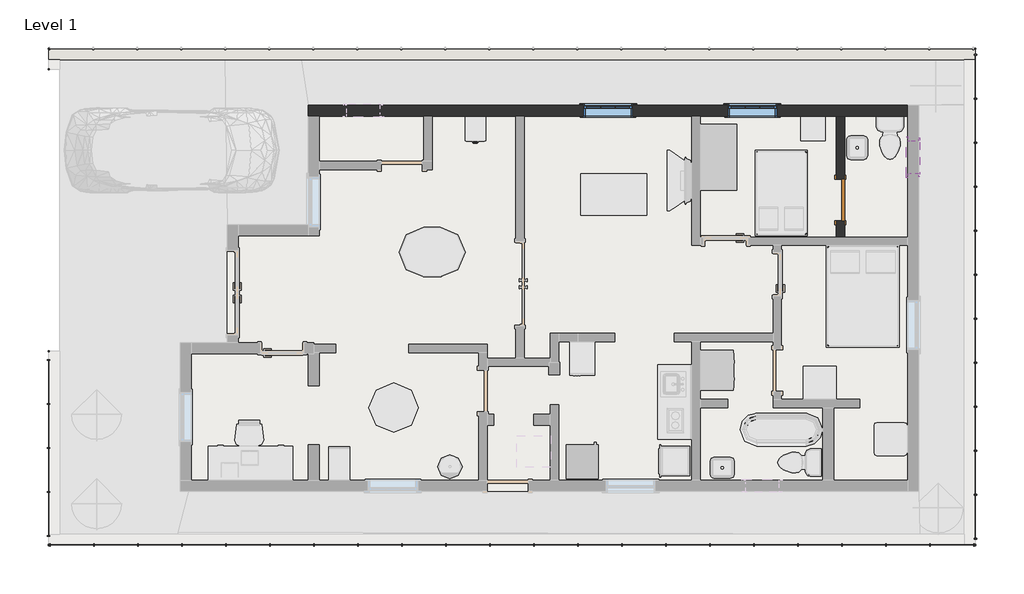
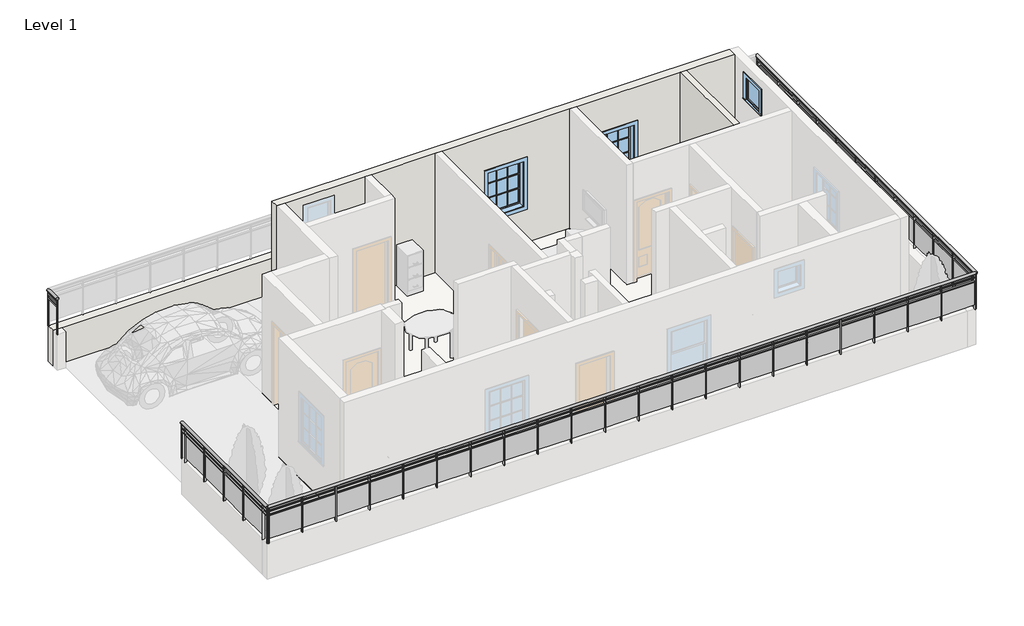
# One storey, part 2 of 3: 4 railings, 3 walls, 3 windows, 1 door, 1 slab.
"""IFC4 building model written with IfcOpenShell, lengths in millimetres."""

from ifc_helpers import new_model, si_unit, point, frame, origin, place, context, project, spatial, polyline, ellipse_curve, trimmed, outline, extrude, faceted_brep, transform, mapped, element, save
from ifc_brep_helpers import plane_surface, extruded_surface, advanced_brep
from components import door_059fdd7e, window_29c06734, window_e41d21a6

model = new_model("IFC4")

# Units and contexts
model_context = context("Model", 3, world=origin())
ifc_project = project(units=[si_unit("LENGTHUNIT", "METRE", prefix="MILLI")], contexts=[model_context])

# Site, building, storey
site = spatial("IfcSite", under=ifc_project)
building = spatial("IfcBuilding", under=site)
storey = spatial("IfcBuildingStorey", under=building, Name="Level 1", Elevation=0.0)

# Door
placement = place(None, origin())
door_shape = door_059fdd7e(model_context)
element("IfcDoor", 1, ObjectType="Single-Flush : 30\" x 80\"", at=placement, inside=storey, context=model_context, shape_type="MappedRepresentation", body=[
    mapped(door_shape, transform((-7474.6845566, 9582.2812219, 0.0), x_axis=(0.0, -1.0, 0.0), y_axis=(1.0, 0.0, 0.0), z_axis=(0.0, 0.0, 1.0))),
])

# Railings
element("IfcRailing", 2, ObjectType="Glass Panel - Bottom Fill", at=placement, inside=storey, context=model_context, shape_type="SolidModel", body=[
    advanced_brep(
    [(-22063.2202606, 6788.8658827, 1828.8), (-22139.4202606, 6788.8658827, 1828.8), (-22063.2202606, 3207.4658827, 1828.8), (-22139.4202606, 3207.4658827, 1828.8)],
    [
        (0, 1, ellipse_curve(frame((-22101.3202606, 6788.8658827, 1828.8), z_axis=(0.0, 1.0, 0.0), x_axis=(-1.0, 0.0, 0.0)), 38.1, 28.575)),
        (1, 0, ellipse_curve(frame((-22101.3202606, 6788.8658827, 1828.8), z_axis=(0.0, 1.0, 0.0), x_axis=(-1.0, 0.0, 0.0)), 38.1, 28.575)),
        (2, 3, ellipse_curve(frame((-22101.3202606, 3207.4658827, 1828.8), z_axis=(0.0, -1.0, 0.0), x_axis=(-1.0, 0.0, 0.0)), 38.1, 28.575)),
        (3, 2, ellipse_curve(frame((-22101.3202606, 3207.4658827, 1828.8), z_axis=(0.0, -1.0, 0.0), x_axis=(-1.0, 0.0, 0.0)), 38.1, 28.575)),
        (0, 2),
        (3, 1),
    ],
    [
        plane_surface(frame((-22101.3202606, 6788.8658827, 1828.8), z_axis=(0.0, 1.0, 0.0), x_axis=(0.0, 0.0, -1.0))),
        plane_surface(frame((-22101.3202606, 3207.4658827, 1828.8), z_axis=(0.0, -1.0, 0.0), x_axis=(0.0, 0.0, -1.0))),
        extruded_surface(trimmed(ellipse_curve(frame((-22101.3202606, 3207.4658827, 1828.8), z_axis=(0.0, 1.0, 0.0), x_axis=(-1.0, 0.0, 0.0)), 38.1, 28.575), [point((-22063.2202606, 3207.4658827, 1828.8))], [point((-22139.4202606, 3207.4658827, 1828.8))], True, "CARTESIAN"), (0.0, 3581.4, 0.0), 3581.4),
        extruded_surface(trimmed(ellipse_curve(frame((-22101.3202606, 3207.4658827, 1828.8), z_axis=(0.0, 1.0, 0.0), x_axis=(-1.0, 0.0, 0.0)), 38.1, 28.575), [point((-22139.4202606, 3207.4658827, 1828.8))], [point((-22063.2202606, 3207.4658827, 1828.8))], True, "CARTESIAN"), (0.0, 3581.4, 0.0), 3581.4),
    ],
    [
        (0, [[1, 2]]),
        (1, [[3, 4]]),
        (2, [[-1, 5, -4, 6]]),
        (3, [[-2, -6, -3, -5]]),
    ],
),
    extrude(outline(polyline([(-22114.0202606, 6788.8658827), (-22088.6202606, 6788.8658827), (-22088.6202606, 3207.4658827), (-22114.0202606, 3207.4658827), (-22114.0202606, 6788.8658827)])), frame((0.0, 0.0, 1714.5), z_axis=(0.0, 0.0, 1.0), x_axis=(1.0, 0.0, 0.0)), (0.0, 0.0, 1.0), 25.4),
    extrude(outline(polyline([(-22114.0202606, 6788.8658827), (-22088.6202606, 6788.8658827), (-22088.6202606, 3207.4658827), (-22114.0202606, 3207.4658827), (-22114.0202606, 6788.8658827)])), frame((0.0, 0.0, 1612.9), z_axis=(0.0, 0.0, 1.0), x_axis=(1.0, 0.0, 0.0)), (0.0, 0.0, 1.0), 25.4),
    extrude(outline(polyline([(-22126.7202606, 3378.9158827), (-22075.9202606, 3378.9158827), (-22075.9202606, 3366.2158827), (-22126.7202606, 3366.2158827), (-22126.7202606, 3378.9158827)])), frame((0.0, 0.0, 914.4), z_axis=(0.0, 0.0, 1.0), x_axis=(1.0, 0.0, 0.0)), (0.0, 0.0, 1.0), 885.6788223),
    extrude(outline(polyline([(-22094.7851036, 4185.3658827), (-22094.7851036, 3372.5658827), (-22101.1351036, 3372.5658827), (-22101.1351036, 4185.3658827), (-22094.7851036, 4185.3658827)])), frame((0.0, 0.0, 1016.0), z_axis=(0.0, 0.0, 1.0), x_axis=(1.0, 0.0, 0.0)), (0.0, 0.0, 1.0), 596.9),
    extrude(outline(polyline([(-22126.7202606, 4191.7158827), (-22075.9202606, 4191.7158827), (-22075.9202606, 4179.0158827), (-22126.7202606, 4179.0158827), (-22126.7202606, 4191.7158827)])), frame((0.0, 0.0, 914.4), z_axis=(0.0, 0.0, 1.0), x_axis=(1.0, 0.0, 0.0)), (0.0, 0.0, 1.0), 885.6788223),
    extrude(outline(polyline([(-22094.7851036, 4998.1658827), (-22094.7851036, 4185.3658827), (-22101.1351036, 4185.3658827), (-22101.1351036, 4998.1658827), (-22094.7851036, 4998.1658827)])), frame((0.0, 0.0, 1016.0), z_axis=(0.0, 0.0, 1.0), x_axis=(1.0, 0.0, 0.0)), (0.0, 0.0, 1.0), 596.9),
    extrude(outline(polyline([(-22126.7202606, 5004.5158827), (-22075.9202606, 5004.5158827), (-22075.9202606, 4991.8158827), (-22126.7202606, 4991.8158827), (-22126.7202606, 5004.5158827)])), frame((0.0, 0.0, 914.4), z_axis=(0.0, 0.0, 1.0), x_axis=(1.0, 0.0, 0.0)), (0.0, 0.0, 1.0), 885.6788223),
    extrude(outline(polyline([(-22094.7851036, 5810.9658827), (-22094.7851036, 4998.1658827), (-22101.1351036, 4998.1658827), (-22101.1351036, 5810.9658827), (-22094.7851036, 5810.9658827)])), frame((0.0, 0.0, 1016.0), z_axis=(0.0, 0.0, 1.0), x_axis=(1.0, 0.0, 0.0)), (0.0, 0.0, 1.0), 596.9),
    extrude(outline(polyline([(-22126.7202606, 5817.3158827), (-22075.9202606, 5817.3158827), (-22075.9202606, 5804.6158827), (-22126.7202606, 5804.6158827), (-22126.7202606, 5817.3158827)])), frame((0.0, 0.0, 914.4), z_axis=(0.0, 0.0, 1.0), x_axis=(1.0, 0.0, 0.0)), (0.0, 0.0, 1.0), 885.6788223),
    extrude(outline(polyline([(-22094.7851036, 6623.7658827), (-22094.7851036, 5810.9658827), (-22101.1351036, 5810.9658827), (-22101.1351036, 6623.7658827), (-22094.7851036, 6623.7658827)])), frame((0.0, 0.0, 1016.0), z_axis=(0.0, 0.0, 1.0), x_axis=(1.0, 0.0, 0.0)), (0.0, 0.0, 1.0), 596.9),
    extrude(outline(polyline([(-22126.7202606, 6630.1158827), (-22075.9202606, 6630.1158827), (-22075.9202606, 6617.4158827), (-22126.7202606, 6617.4158827), (-22126.7202606, 6630.1158827)])), frame((0.0, 0.0, 914.4), z_axis=(0.0, 0.0, 1.0), x_axis=(1.0, 0.0, 0.0)), (0.0, 0.0, 1.0), 885.6788223),
    extrude(outline(polyline([(-22110.8452606, 3220.1658827), (-22091.7952606, 3220.1658827), (-22091.7952606, 3201.1158827), (-22110.8452606, 3201.1158827), (-22110.8452606, 3220.1658827)])), frame((0.0, 0.0, 914.4), z_axis=(0.0, 0.0, 1.0), x_axis=(1.0, 0.0, 0.0)), (0.0, 0.0, 1.0), 885.6788223),
    extrude(outline(polyline([(-22110.8452606, 6795.2158827), (-22091.7952606, 6795.2158827), (-22091.7952606, 6776.1658827), (-22110.8452606, 6776.1658827), (-22110.8452606, 6795.2158827)])), frame((0.0, 0.0, 914.4), z_axis=(0.0, 0.0, 1.0), x_axis=(1.0, 0.0, 0.0)), (0.0, 0.0, 1.0), 885.6788223),
])
element("IfcRailing", 3, ObjectType="Glass Panel - Bottom Fill", at=placement, inside=storey, context=model_context, shape_type="SolidModel", body=[
    advanced_brep(
    [(-22101.3202606, 3245.5658827, 1828.8), (-22101.3202606, 3169.3658827, 1828.8), (-4981.7202606, 3245.5658827, 1828.8), (-4981.7202606, 3169.3658827, 1828.8)],
    [
        (0, 1, ellipse_curve(frame((-22101.3202606, 3207.4658827, 1828.8), z_axis=(-1.0, 0.0, 0.0), x_axis=(0.0, -1.0, 0.0)), 38.1, 28.575)),
        (1, 0, ellipse_curve(frame((-22101.3202606, 3207.4658827, 1828.8), z_axis=(-1.0, 0.0, 0.0), x_axis=(0.0, -1.0, 0.0)), 38.1, 28.575)),
        (2, 3, ellipse_curve(frame((-4981.7202606, 3207.4658827, 1828.8), z_axis=(1.0, 0.0, 0.0), x_axis=(0.0, -1.0, 0.0)), 38.1, 28.575)),
        (3, 2, ellipse_curve(frame((-4981.7202606, 3207.4658827, 1828.8), z_axis=(1.0, 0.0, 0.0), x_axis=(0.0, -1.0, 0.0)), 38.1, 28.575)),
        (0, 2),
        (3, 1),
    ],
    [
        plane_surface(frame((-22101.3202606, 3207.4658827, 1828.8), z_axis=(-1.0, 0.0, 0.0), x_axis=(0.0, 1.0, 0.0))),
        plane_surface(frame((-4981.7202606, 3207.4658827, 1828.8), z_axis=(1.0, 0.0, 0.0), x_axis=(0.0, 1.0, 0.0))),
        extruded_surface(trimmed(ellipse_curve(frame((-4981.7202606, 3207.4658827, 1828.8), z_axis=(-1.0, 0.0, 0.0), x_axis=(0.0, -1.0, 0.0)), 38.1, 28.575), [point((-4981.7202606, 3245.5658827, 1828.8))], [point((-4981.7202606, 3169.3658827, 1828.8))], True, "CARTESIAN"), (-17119.600000000002, 0.0, 0.0), 17119.600000000002),
        extruded_surface(trimmed(ellipse_curve(frame((-4981.7202606, 3207.4658827, 1828.8), z_axis=(-1.0, 0.0, 0.0), x_axis=(0.0, -1.0, 0.0)), 38.1, 28.575), [point((-4981.7202606, 3169.3658827, 1828.8))], [point((-4981.7202606, 3245.5658827, 1828.8))], True, "CARTESIAN"), (-17119.600000000002, 0.0, 0.0), 17119.600000000002),
    ],
    [
        (0, [[1, 2]]),
        (1, [[3, 4]]),
        (2, [[-1, 5, -4, 6]]),
        (3, [[-2, -6, -3, -5]]),
    ],
),
    extrude(outline(polyline([(-22101.3202606, 3194.7658827), (-22101.3202606, 3220.1658827), (-4981.7202606, 3220.1658827), (-4981.7202606, 3194.7658827), (-22101.3202606, 3194.7658827)])), frame((0.0, 0.0, 1714.5), z_axis=(0.0, 0.0, 1.0), x_axis=(1.0, 0.0, 0.0)), (0.0, 0.0, 1.0), 25.4),
    extrude(outline(polyline([(-22101.3202606, 3194.7658827), (-22101.3202606, 3220.1658827), (-4981.7202606, 3220.1658827), (-4981.7202606, 3194.7658827), (-22101.3202606, 3194.7658827)])), frame((0.0, 0.0, 1612.9), z_axis=(0.0, 0.0, 1.0), x_axis=(1.0, 0.0, 0.0)), (0.0, 0.0, 1.0), 25.4),
    extrude(outline(polyline([(-5013.4702606, 3182.0658827), (-5013.4702606, 3232.8658827), (-5000.7702606, 3232.8658827), (-5000.7702606, 3182.0658827), (-5013.4702606, 3182.0658827)])), frame((0.0, 0.0, 914.4), z_axis=(0.0, 0.0, 1.0), x_axis=(1.0, 0.0, 0.0)), (0.0, 0.0, 1.0), 885.6788223),
    extrude(outline(polyline([(-5819.9202606, 3214.0010397), (-5007.1202606, 3214.0010397), (-5007.1202606, 3207.6510397), (-5819.9202606, 3207.6510397), (-5819.9202606, 3214.0010397)])), frame((0.0, 0.0, 1016.0), z_axis=(0.0, 0.0, 1.0), x_axis=(1.0, 0.0, 0.0)), (0.0, 0.0, 1.0), 596.9),
    extrude(outline(polyline([(-5826.2702606, 3182.0658827), (-5826.2702606, 3232.8658827), (-5813.5702606, 3232.8658827), (-5813.5702606, 3182.0658827), (-5826.2702606, 3182.0658827)])), frame((0.0, 0.0, 914.4), z_axis=(0.0, 0.0, 1.0), x_axis=(1.0, 0.0, 0.0)), (0.0, 0.0, 1.0), 885.6788223),
    extrude(outline(polyline([(-6632.7202606, 3214.0010397), (-5819.9202606, 3214.0010397), (-5819.9202606, 3207.6510397), (-6632.7202606, 3207.6510397), (-6632.7202606, 3214.0010397)])), frame((0.0, 0.0, 1016.0), z_axis=(0.0, 0.0, 1.0), x_axis=(1.0, 0.0, 0.0)), (0.0, 0.0, 1.0), 596.9),
    extrude(outline(polyline([(-6639.0702606, 3182.0658827), (-6639.0702606, 3232.8658827), (-6626.3702606, 3232.8658827), (-6626.3702606, 3182.0658827), (-6639.0702606, 3182.0658827)])), frame((0.0, 0.0, 914.4), z_axis=(0.0, 0.0, 1.0), x_axis=(1.0, 0.0, 0.0)), (0.0, 0.0, 1.0), 885.6788223),
    extrude(outline(polyline([(-7445.5202606, 3214.0010397), (-6632.7202606, 3214.0010397), (-6632.7202606, 3207.6510397), (-7445.5202606, 3207.6510397), (-7445.5202606, 3214.0010397)])), frame((0.0, 0.0, 1016.0), z_axis=(0.0, 0.0, 1.0), x_axis=(1.0, 0.0, 0.0)), (0.0, 0.0, 1.0), 596.9),
    extrude(outline(polyline([(-7451.8702606, 3182.0658827), (-7451.8702606, 3232.8658827), (-7439.1702606, 3232.8658827), (-7439.1702606, 3182.0658827), (-7451.8702606, 3182.0658827)])), frame((0.0, 0.0, 914.4), z_axis=(0.0, 0.0, 1.0), x_axis=(1.0, 0.0, 0.0)), (0.0, 0.0, 1.0), 885.6788223),
    extrude(outline(polyline([(-8258.3202606, 3214.0010397), (-7445.5202606, 3214.0010397), (-7445.5202606, 3207.6510397), (-8258.3202606, 3207.6510397), (-8258.3202606, 3214.0010397)])), frame((0.0, 0.0, 1016.0), z_axis=(0.0, 0.0, 1.0), x_axis=(1.0, 0.0, 0.0)), (0.0, 0.0, 1.0), 596.9),
    extrude(outline(polyline([(-8264.6702606, 3182.0658827), (-8264.6702606, 3232.8658827), (-8251.9702606, 3232.8658827), (-8251.9702606, 3182.0658827), (-8264.6702606, 3182.0658827)])), frame((0.0, 0.0, 914.4), z_axis=(0.0, 0.0, 1.0), x_axis=(1.0, 0.0, 0.0)), (0.0, 0.0, 1.0), 885.6788223),
    extrude(outline(polyline([(-9071.1202606, 3214.0010397), (-8258.3202606, 3214.0010397), (-8258.3202606, 3207.6510397), (-9071.1202606, 3207.6510397), (-9071.1202606, 3214.0010397)])), frame((0.0, 0.0, 1016.0), z_axis=(0.0, 0.0, 1.0), x_axis=(1.0, 0.0, 0.0)), (0.0, 0.0, 1.0), 596.9),
    extrude(outline(polyline([(-9077.4702606, 3182.0658827), (-9077.4702606, 3232.8658827), (-9064.7702606, 3232.8658827), (-9064.7702606, 3182.0658827), (-9077.4702606, 3182.0658827)])), frame((0.0, 0.0, 914.4), z_axis=(0.0, 0.0, 1.0), x_axis=(1.0, 0.0, 0.0)), (0.0, 0.0, 1.0), 885.6788223),
    extrude(outline(polyline([(-9883.9202606, 3214.0010397), (-9071.1202606, 3214.0010397), (-9071.1202606, 3207.6510397), (-9883.9202606, 3207.6510397), (-9883.9202606, 3214.0010397)])), frame((0.0, 0.0, 1016.0), z_axis=(0.0, 0.0, 1.0), x_axis=(1.0, 0.0, 0.0)), (0.0, 0.0, 1.0), 596.9),
    extrude(outline(polyline([(-9890.2702606, 3182.0658827), (-9890.2702606, 3232.8658827), (-9877.5702606, 3232.8658827), (-9877.5702606, 3182.0658827), (-9890.2702606, 3182.0658827)])), frame((0.0, 0.0, 914.4), z_axis=(0.0, 0.0, 1.0), x_axis=(1.0, 0.0, 0.0)), (0.0, 0.0, 1.0), 885.6788223),
    extrude(outline(polyline([(-10696.7202606, 3214.0010397), (-9883.9202606, 3214.0010397), (-9883.9202606, 3207.6510397), (-10696.7202606, 3207.6510397), (-10696.7202606, 3214.0010397)])), frame((0.0, 0.0, 1016.0), z_axis=(0.0, 0.0, 1.0), x_axis=(1.0, 0.0, 0.0)), (0.0, 0.0, 1.0), 596.9),
    extrude(outline(polyline([(-10703.0702606, 3182.0658827), (-10703.0702606, 3232.8658827), (-10690.3702606, 3232.8658827), (-10690.3702606, 3182.0658827), (-10703.0702606, 3182.0658827)])), frame((0.0, 0.0, 914.4), z_axis=(0.0, 0.0, 1.0), x_axis=(1.0, 0.0, 0.0)), (0.0, 0.0, 1.0), 885.6788223),
    extrude(outline(polyline([(-11509.5202606, 3214.0010397), (-10696.7202606, 3214.0010397), (-10696.7202606, 3207.6510397), (-11509.5202606, 3207.6510397), (-11509.5202606, 3214.0010397)])), frame((0.0, 0.0, 1016.0), z_axis=(0.0, 0.0, 1.0), x_axis=(1.0, 0.0, 0.0)), (0.0, 0.0, 1.0), 596.9),
    extrude(outline(polyline([(-11515.8702606, 3182.0658827), (-11515.8702606, 3232.8658827), (-11503.1702606, 3232.8658827), (-11503.1702606, 3182.0658827), (-11515.8702606, 3182.0658827)])), frame((0.0, 0.0, 914.4), z_axis=(0.0, 0.0, 1.0), x_axis=(1.0, 0.0, 0.0)), (0.0, 0.0, 1.0), 885.6788223),
    extrude(outline(polyline([(-12322.3202606, 3214.0010397), (-11509.5202606, 3214.0010397), (-11509.5202606, 3207.6510397), (-12322.3202606, 3207.6510397), (-12322.3202606, 3214.0010397)])), frame((0.0, 0.0, 1016.0), z_axis=(0.0, 0.0, 1.0), x_axis=(1.0, 0.0, 0.0)), (0.0, 0.0, 1.0), 596.9),
    extrude(outline(polyline([(-12328.6702606, 3182.0658827), (-12328.6702606, 3232.8658827), (-12315.9702606, 3232.8658827), (-12315.9702606, 3182.0658827), (-12328.6702606, 3182.0658827)])), frame((0.0, 0.0, 914.4), z_axis=(0.0, 0.0, 1.0), x_axis=(1.0, 0.0, 0.0)), (0.0, 0.0, 1.0), 885.6788223),
    extrude(outline(polyline([(-13135.1202606, 3214.0010397), (-12322.3202606, 3214.0010397), (-12322.3202606, 3207.6510397), (-13135.1202606, 3207.6510397), (-13135.1202606, 3214.0010397)])), frame((0.0, 0.0, 1016.0), z_axis=(0.0, 0.0, 1.0), x_axis=(1.0, 0.0, 0.0)), (0.0, 0.0, 1.0), 596.9),
    extrude(outline(polyline([(-13141.4702606, 3182.0658827), (-13141.4702606, 3232.8658827), (-13128.7702606, 3232.8658827), (-13128.7702606, 3182.0658827), (-13141.4702606, 3182.0658827)])), frame((0.0, 0.0, 914.4), z_axis=(0.0, 0.0, 1.0), x_axis=(1.0, 0.0, 0.0)), (0.0, 0.0, 1.0), 885.6788223),
    extrude(outline(polyline([(-13947.9202606, 3214.0010397), (-13135.1202606, 3214.0010397), (-13135.1202606, 3207.6510397), (-13947.9202606, 3207.6510397), (-13947.9202606, 3214.0010397)])), frame((0.0, 0.0, 1016.0), z_axis=(0.0, 0.0, 1.0), x_axis=(1.0, 0.0, 0.0)), (0.0, 0.0, 1.0), 596.9),
    extrude(outline(polyline([(-13954.2702606, 3182.0658827), (-13954.2702606, 3232.8658827), (-13941.5702606, 3232.8658827), (-13941.5702606, 3182.0658827), (-13954.2702606, 3182.0658827)])), frame((0.0, 0.0, 914.4), z_axis=(0.0, 0.0, 1.0), x_axis=(1.0, 0.0, 0.0)), (0.0, 0.0, 1.0), 885.6788223),
    extrude(outline(polyline([(-14760.7202606, 3214.0010397), (-13947.9202606, 3214.0010397), (-13947.9202606, 3207.6510397), (-14760.7202606, 3207.6510397), (-14760.7202606, 3214.0010397)])), frame((0.0, 0.0, 1016.0), z_axis=(0.0, 0.0, 1.0), x_axis=(1.0, 0.0, 0.0)), (0.0, 0.0, 1.0), 596.9),
    extrude(outline(polyline([(-14767.0702606, 3182.0658827), (-14767.0702606, 3232.8658827), (-14754.3702606, 3232.8658827), (-14754.3702606, 3182.0658827), (-14767.0702606, 3182.0658827)])), frame((0.0, 0.0, 914.4), z_axis=(0.0, 0.0, 1.0), x_axis=(1.0, 0.0, 0.0)), (0.0, 0.0, 1.0), 885.6788223),
    extrude(outline(polyline([(-15573.5202606, 3214.0010397), (-14760.7202606, 3214.0010397), (-14760.7202606, 3207.6510397), (-15573.5202606, 3207.6510397), (-15573.5202606, 3214.0010397)])), frame((0.0, 0.0, 1016.0), z_axis=(0.0, 0.0, 1.0), x_axis=(1.0, 0.0, 0.0)), (0.0, 0.0, 1.0), 596.9),
    extrude(outline(polyline([(-15579.8702606, 3182.0658827), (-15579.8702606, 3232.8658827), (-15567.1702606, 3232.8658827), (-15567.1702606, 3182.0658827), (-15579.8702606, 3182.0658827)])), frame((0.0, 0.0, 914.4), z_axis=(0.0, 0.0, 1.0), x_axis=(1.0, 0.0, 0.0)), (0.0, 0.0, 1.0), 885.6788223),
    extrude(outline(polyline([(-16386.3202606, 3214.0010397), (-15573.5202606, 3214.0010397), (-15573.5202606, 3207.6510397), (-16386.3202606, 3207.6510397), (-16386.3202606, 3214.0010397)])), frame((0.0, 0.0, 1016.0), z_axis=(0.0, 0.0, 1.0), x_axis=(1.0, 0.0, 0.0)), (0.0, 0.0, 1.0), 596.9),
    extrude(outline(polyline([(-16392.6702606, 3182.0658827), (-16392.6702606, 3232.8658827), (-16379.9702606, 3232.8658827), (-16379.9702606, 3182.0658827), (-16392.6702606, 3182.0658827)])), frame((0.0, 0.0, 914.4), z_axis=(0.0, 0.0, 1.0), x_axis=(1.0, 0.0, 0.0)), (0.0, 0.0, 1.0), 885.6788223),
    extrude(outline(polyline([(-17199.1202606, 3214.0010397), (-16386.3202606, 3214.0010397), (-16386.3202606, 3207.6510397), (-17199.1202606, 3207.6510397), (-17199.1202606, 3214.0010397)])), frame((0.0, 0.0, 1016.0), z_axis=(0.0, 0.0, 1.0), x_axis=(1.0, 0.0, 0.0)), (0.0, 0.0, 1.0), 596.9),
    extrude(outline(polyline([(-17205.4702606, 3182.0658827), (-17205.4702606, 3232.8658827), (-17192.7702606, 3232.8658827), (-17192.7702606, 3182.0658827), (-17205.4702606, 3182.0658827)])), frame((0.0, 0.0, 914.4), z_axis=(0.0, 0.0, 1.0), x_axis=(1.0, 0.0, 0.0)), (0.0, 0.0, 1.0), 885.6788223),
    extrude(outline(polyline([(-18011.9202606, 3214.0010397), (-17199.1202606, 3214.0010397), (-17199.1202606, 3207.6510397), (-18011.9202606, 3207.6510397), (-18011.9202606, 3214.0010397)])), frame((0.0, 0.0, 1016.0), z_axis=(0.0, 0.0, 1.0), x_axis=(1.0, 0.0, 0.0)), (0.0, 0.0, 1.0), 596.9),
    extrude(outline(polyline([(-18018.2702606, 3182.0658827), (-18018.2702606, 3232.8658827), (-18005.5702606, 3232.8658827), (-18005.5702606, 3182.0658827), (-18018.2702606, 3182.0658827)])), frame((0.0, 0.0, 914.4), z_axis=(0.0, 0.0, 1.0), x_axis=(1.0, 0.0, 0.0)), (0.0, 0.0, 1.0), 885.6788223),
    extrude(outline(polyline([(-18824.7202606, 3214.0010397), (-18011.9202606, 3214.0010397), (-18011.9202606, 3207.6510397), (-18824.7202606, 3207.6510397), (-18824.7202606, 3214.0010397)])), frame((0.0, 0.0, 1016.0), z_axis=(0.0, 0.0, 1.0), x_axis=(1.0, 0.0, 0.0)), (0.0, 0.0, 1.0), 596.9),
    extrude(outline(polyline([(-18831.0702606, 3182.0658827), (-18831.0702606, 3232.8658827), (-18818.3702606, 3232.8658827), (-18818.3702606, 3182.0658827), (-18831.0702606, 3182.0658827)])), frame((0.0, 0.0, 914.4), z_axis=(0.0, 0.0, 1.0), x_axis=(1.0, 0.0, 0.0)), (0.0, 0.0, 1.0), 885.6788223),
    extrude(outline(polyline([(-19637.5202606, 3214.0010397), (-18824.7202606, 3214.0010397), (-18824.7202606, 3207.6510397), (-19637.5202606, 3207.6510397), (-19637.5202606, 3214.0010397)])), frame((0.0, 0.0, 1016.0), z_axis=(0.0, 0.0, 1.0), x_axis=(1.0, 0.0, 0.0)), (0.0, 0.0, 1.0), 596.9),
    extrude(outline(polyline([(-19643.8702606, 3182.0658827), (-19643.8702606, 3232.8658827), (-19631.1702606, 3232.8658827), (-19631.1702606, 3182.0658827), (-19643.8702606, 3182.0658827)])), frame((0.0, 0.0, 914.4), z_axis=(0.0, 0.0, 1.0), x_axis=(1.0, 0.0, 0.0)), (0.0, 0.0, 1.0), 885.6788223),
    extrude(outline(polyline([(-20450.3202606, 3214.0010397), (-19637.5202606, 3214.0010397), (-19637.5202606, 3207.6510397), (-20450.3202606, 3207.6510397), (-20450.3202606, 3214.0010397)])), frame((0.0, 0.0, 1016.0), z_axis=(0.0, 0.0, 1.0), x_axis=(1.0, 0.0, 0.0)), (0.0, 0.0, 1.0), 596.9),
    extrude(outline(polyline([(-20456.6702606, 3182.0658827), (-20456.6702606, 3232.8658827), (-20443.9702606, 3232.8658827), (-20443.9702606, 3182.0658827), (-20456.6702606, 3182.0658827)])), frame((0.0, 0.0, 914.4), z_axis=(0.0, 0.0, 1.0), x_axis=(1.0, 0.0, 0.0)), (0.0, 0.0, 1.0), 885.6788223),
    extrude(outline(polyline([(-21263.1202606, 3214.0010397), (-20450.3202606, 3214.0010397), (-20450.3202606, 3207.6510397), (-21263.1202606, 3207.6510397), (-21263.1202606, 3214.0010397)])), frame((0.0, 0.0, 1016.0), z_axis=(0.0, 0.0, 1.0), x_axis=(1.0, 0.0, 0.0)), (0.0, 0.0, 1.0), 596.9),
    extrude(outline(polyline([(-21269.4702606, 3182.0658827), (-21269.4702606, 3232.8658827), (-21256.7702606, 3232.8658827), (-21256.7702606, 3182.0658827), (-21269.4702606, 3182.0658827)])), frame((0.0, 0.0, 914.4), z_axis=(0.0, 0.0, 1.0), x_axis=(1.0, 0.0, 0.0)), (0.0, 0.0, 1.0), 885.6788223),
    extrude(outline(polyline([(-22075.9202606, 3214.0010397), (-21263.1202606, 3214.0010397), (-21263.1202606, 3207.6510397), (-22075.9202606, 3207.6510397), (-22075.9202606, 3214.0010397)])), frame((0.0, 0.0, 1016.0), z_axis=(0.0, 0.0, 1.0), x_axis=(1.0, 0.0, 0.0)), (0.0, 0.0, 1.0), 596.9),
    extrude(outline(polyline([(-22082.2702606, 3182.0658827), (-22082.2702606, 3232.8658827), (-22069.5702606, 3232.8658827), (-22069.5702606, 3182.0658827), (-22082.2702606, 3182.0658827)])), frame((0.0, 0.0, 914.4), z_axis=(0.0, 0.0, 1.0), x_axis=(1.0, 0.0, 0.0)), (0.0, 0.0, 1.0), 885.6788223),
    extrude(outline(polyline([(-4994.4202606, 3197.9408827), (-4994.4202606, 3216.9908827), (-4975.3702606, 3216.9908827), (-4975.3702606, 3197.9408827), (-4994.4202606, 3197.9408827)])), frame((0.0, 0.0, 914.4), z_axis=(0.0, 0.0, 1.0), x_axis=(1.0, 0.0, 0.0)), (0.0, 0.0, 1.0), 885.6788223),
    extrude(outline(polyline([(-22107.6702606, 3197.9408827), (-22107.6702606, 3216.9908827), (-22088.6202606, 3216.9908827), (-22088.6202606, 3197.9408827), (-22107.6702606, 3197.9408827)])), frame((0.0, 0.0, 914.4), z_axis=(0.0, 0.0, 1.0), x_axis=(1.0, 0.0, 0.0)), (0.0, 0.0, 1.0), 885.6788223),
])
element("IfcRailing", 4, ObjectType="Glass Panel - Bottom Fill", at=placement, inside=storey, context=model_context, shape_type="SolidModel", body=[
    advanced_brep(
    [(-5019.8202606, 3207.4658827, 1828.8), (-4943.6202606, 3207.4658827, 1828.8), (-5019.8202606, 12376.8658827, 1828.8), (-4943.6202606, 12376.8658827, 1828.8)],
    [
        (0, 1, ellipse_curve(frame((-4981.7202606, 3207.4658827, 1828.8), z_axis=(0.0, -1.0, 0.0), x_axis=(1.0, 0.0, 0.0)), 38.1, 28.575)),
        (1, 0, ellipse_curve(frame((-4981.7202606, 3207.4658827, 1828.8), z_axis=(0.0, -1.0, 0.0), x_axis=(1.0, 0.0, 0.0)), 38.1, 28.575)),
        (2, 3, ellipse_curve(frame((-4981.7202606, 12376.8658827, 1828.8), z_axis=(0.0, 1.0, 0.0), x_axis=(1.0, 0.0, 0.0)), 38.1, 28.575)),
        (3, 2, ellipse_curve(frame((-4981.7202606, 12376.8658827, 1828.8), z_axis=(0.0, 1.0, 0.0), x_axis=(1.0, 0.0, 0.0)), 38.1, 28.575)),
        (0, 2),
        (3, 1),
    ],
    [
        plane_surface(frame((-4981.7202606, 3207.4658827, 1828.8), z_axis=(0.0, -1.0, 0.0), x_axis=(0.0, 0.0, 1.0))),
        plane_surface(frame((-4981.7202606, 12376.8658827, 1828.8), z_axis=(0.0, 1.0, 0.0), x_axis=(0.0, 0.0, 1.0))),
        extruded_surface(trimmed(ellipse_curve(frame((-4981.7202606, 12376.8658827, 1828.8), z_axis=(0.0, -1.0, 0.0), x_axis=(1.0, 0.0, 0.0)), 38.1, 28.575), [point((-5019.8202606, 12376.8658827, 1828.8))], [point((-4943.6202606, 12376.8658827, 1828.8))], True, "CARTESIAN"), (0.0, -9169.4, 0.0), 9169.4),
        extruded_surface(trimmed(ellipse_curve(frame((-4981.7202606, 12376.8658827, 1828.8), z_axis=(0.0, -1.0, 0.0), x_axis=(1.0, 0.0, 0.0)), 38.1, 28.575), [point((-4943.6202606, 12376.8658827, 1828.8))], [point((-5019.8202606, 12376.8658827, 1828.8))], True, "CARTESIAN"), (0.0, -9169.4, 0.0), 9169.4),
    ],
    [
        (0, [[1, 2]]),
        (1, [[3, 4]]),
        (2, [[-1, 5, -4, 6]]),
        (3, [[-2, -6, -3, -5]]),
    ],
),
    extrude(outline(polyline([(-4969.0202606, 3207.4658827), (-4994.4202606, 3207.4658827), (-4994.4202606, 12376.8658827), (-4969.0202606, 12376.8658827), (-4969.0202606, 3207.4658827)])), frame((0.0, 0.0, 1714.5), z_axis=(0.0, 0.0, 1.0), x_axis=(1.0, 0.0, 0.0)), (0.0, 0.0, 1.0), 25.4),
    extrude(outline(polyline([(-4969.0202606, 3207.4658827), (-4994.4202606, 3207.4658827), (-4994.4202606, 12376.8658827), (-4969.0202606, 12376.8658827), (-4969.0202606, 3207.4658827)])), frame((0.0, 0.0, 1612.9), z_axis=(0.0, 0.0, 1.0), x_axis=(1.0, 0.0, 0.0)), (0.0, 0.0, 1.0), 25.4),
    extrude(outline(polyline([(-4956.3202606, 12256.2158827), (-5007.1202606, 12256.2158827), (-5007.1202606, 12268.9158827), (-4956.3202606, 12268.9158827), (-4956.3202606, 12256.2158827)])), frame((0.0, 0.0, 914.4), z_axis=(0.0, 0.0, 1.0), x_axis=(1.0, 0.0, 0.0)), (0.0, 0.0, 1.0), 885.6788223),
    extrude(outline(polyline([(-4988.2554176, 11449.7658827), (-4988.2554176, 12262.5658827), (-4981.9054176, 12262.5658827), (-4981.9054176, 11449.7658827), (-4988.2554176, 11449.7658827)])), frame((0.0, 0.0, 1016.0), z_axis=(0.0, 0.0, 1.0), x_axis=(1.0, 0.0, 0.0)), (0.0, 0.0, 1.0), 596.9),
    extrude(outline(polyline([(-4956.3202606, 11443.4158827), (-5007.1202606, 11443.4158827), (-5007.1202606, 11456.1158827), (-4956.3202606, 11456.1158827), (-4956.3202606, 11443.4158827)])), frame((0.0, 0.0, 914.4), z_axis=(0.0, 0.0, 1.0), x_axis=(1.0, 0.0, 0.0)), (0.0, 0.0, 1.0), 885.6788223),
    extrude(outline(polyline([(-4988.2554176, 10636.9658827), (-4988.2554176, 11449.7658827), (-4981.9054176, 11449.7658827), (-4981.9054176, 10636.9658827), (-4988.2554176, 10636.9658827)])), frame((0.0, 0.0, 1016.0), z_axis=(0.0, 0.0, 1.0), x_axis=(1.0, 0.0, 0.0)), (0.0, 0.0, 1.0), 596.9),
    extrude(outline(polyline([(-4956.3202606, 10630.6158827), (-5007.1202606, 10630.6158827), (-5007.1202606, 10643.3158827), (-4956.3202606, 10643.3158827), (-4956.3202606, 10630.6158827)])), frame((0.0, 0.0, 914.4), z_axis=(0.0, 0.0, 1.0), x_axis=(1.0, 0.0, 0.0)), (0.0, 0.0, 1.0), 885.6788223),
    extrude(outline(polyline([(-4988.2554176, 9824.1658827), (-4988.2554176, 10636.9658827), (-4981.9054176, 10636.9658827), (-4981.9054176, 9824.1658827), (-4988.2554176, 9824.1658827)])), frame((0.0, 0.0, 1016.0), z_axis=(0.0, 0.0, 1.0), x_axis=(1.0, 0.0, 0.0)), (0.0, 0.0, 1.0), 596.9),
    extrude(outline(polyline([(-4956.3202606, 9817.8158827), (-5007.1202606, 9817.8158827), (-5007.1202606, 9830.5158827), (-4956.3202606, 9830.5158827), (-4956.3202606, 9817.8158827)])), frame((0.0, 0.0, 914.4), z_axis=(0.0, 0.0, 1.0), x_axis=(1.0, 0.0, 0.0)), (0.0, 0.0, 1.0), 885.6788223),
    extrude(outline(polyline([(-4988.2554176, 9011.3658827), (-4988.2554176, 9824.1658827), (-4981.9054176, 9824.1658827), (-4981.9054176, 9011.3658827), (-4988.2554176, 9011.3658827)])), frame((0.0, 0.0, 1016.0), z_axis=(0.0, 0.0, 1.0), x_axis=(1.0, 0.0, 0.0)), (0.0, 0.0, 1.0), 596.9),
    extrude(outline(polyline([(-4956.3202606, 9005.0158827), (-5007.1202606, 9005.0158827), (-5007.1202606, 9017.7158827), (-4956.3202606, 9017.7158827), (-4956.3202606, 9005.0158827)])), frame((0.0, 0.0, 914.4), z_axis=(0.0, 0.0, 1.0), x_axis=(1.0, 0.0, 0.0)), (0.0, 0.0, 1.0), 885.6788223),
    extrude(outline(polyline([(-4988.2554176, 8198.5658827), (-4988.2554176, 9011.3658827), (-4981.9054176, 9011.3658827), (-4981.9054176, 8198.5658827), (-4988.2554176, 8198.5658827)])), frame((0.0, 0.0, 1016.0), z_axis=(0.0, 0.0, 1.0), x_axis=(1.0, 0.0, 0.0)), (0.0, 0.0, 1.0), 596.9),
    extrude(outline(polyline([(-4956.3202606, 8192.2158827), (-5007.1202606, 8192.2158827), (-5007.1202606, 8204.9158827), (-4956.3202606, 8204.9158827), (-4956.3202606, 8192.2158827)])), frame((0.0, 0.0, 914.4), z_axis=(0.0, 0.0, 1.0), x_axis=(1.0, 0.0, 0.0)), (0.0, 0.0, 1.0), 885.6788223),
    extrude(outline(polyline([(-4988.2554176, 7385.7658827), (-4988.2554176, 8198.5658827), (-4981.9054176, 8198.5658827), (-4981.9054176, 7385.7658827), (-4988.2554176, 7385.7658827)])), frame((0.0, 0.0, 1016.0), z_axis=(0.0, 0.0, 1.0), x_axis=(1.0, 0.0, 0.0)), (0.0, 0.0, 1.0), 596.9),
    extrude(outline(polyline([(-4956.3202606, 7379.4158827), (-5007.1202606, 7379.4158827), (-5007.1202606, 7392.1158827), (-4956.3202606, 7392.1158827), (-4956.3202606, 7379.4158827)])), frame((0.0, 0.0, 914.4), z_axis=(0.0, 0.0, 1.0), x_axis=(1.0, 0.0, 0.0)), (0.0, 0.0, 1.0), 885.6788223),
    extrude(outline(polyline([(-4988.2554176, 6572.9658827), (-4988.2554176, 7385.7658827), (-4981.9054176, 7385.7658827), (-4981.9054176, 6572.9658827), (-4988.2554176, 6572.9658827)])), frame((0.0, 0.0, 1016.0), z_axis=(0.0, 0.0, 1.0), x_axis=(1.0, 0.0, 0.0)), (0.0, 0.0, 1.0), 596.9),
    extrude(outline(polyline([(-4956.3202606, 6566.6158827), (-5007.1202606, 6566.6158827), (-5007.1202606, 6579.3158827), (-4956.3202606, 6579.3158827), (-4956.3202606, 6566.6158827)])), frame((0.0, 0.0, 914.4), z_axis=(0.0, 0.0, 1.0), x_axis=(1.0, 0.0, 0.0)), (0.0, 0.0, 1.0), 885.6788223),
    extrude(outline(polyline([(-4988.2554176, 5760.1658827), (-4988.2554176, 6572.9658827), (-4981.9054176, 6572.9658827), (-4981.9054176, 5760.1658827), (-4988.2554176, 5760.1658827)])), frame((0.0, 0.0, 1016.0), z_axis=(0.0, 0.0, 1.0), x_axis=(1.0, 0.0, 0.0)), (0.0, 0.0, 1.0), 596.9),
    extrude(outline(polyline([(-4956.3202606, 5753.8158827), (-5007.1202606, 5753.8158827), (-5007.1202606, 5766.5158827), (-4956.3202606, 5766.5158827), (-4956.3202606, 5753.8158827)])), frame((0.0, 0.0, 914.4), z_axis=(0.0, 0.0, 1.0), x_axis=(1.0, 0.0, 0.0)), (0.0, 0.0, 1.0), 885.6788223),
    extrude(outline(polyline([(-4988.2554176, 4947.3658827), (-4988.2554176, 5760.1658827), (-4981.9054176, 5760.1658827), (-4981.9054176, 4947.3658827), (-4988.2554176, 4947.3658827)])), frame((0.0, 0.0, 1016.0), z_axis=(0.0, 0.0, 1.0), x_axis=(1.0, 0.0, 0.0)), (0.0, 0.0, 1.0), 596.9),
    extrude(outline(polyline([(-4956.3202606, 4941.0158827), (-5007.1202606, 4941.0158827), (-5007.1202606, 4953.7158827), (-4956.3202606, 4953.7158827), (-4956.3202606, 4941.0158827)])), frame((0.0, 0.0, 914.4), z_axis=(0.0, 0.0, 1.0), x_axis=(1.0, 0.0, 0.0)), (0.0, 0.0, 1.0), 885.6788223),
    extrude(outline(polyline([(-4988.2554176, 4134.5658827), (-4988.2554176, 4947.3658827), (-4981.9054176, 4947.3658827), (-4981.9054176, 4134.5658827), (-4988.2554176, 4134.5658827)])), frame((0.0, 0.0, 1016.0), z_axis=(0.0, 0.0, 1.0), x_axis=(1.0, 0.0, 0.0)), (0.0, 0.0, 1.0), 596.9),
    extrude(outline(polyline([(-4956.3202606, 4128.2158827), (-5007.1202606, 4128.2158827), (-5007.1202606, 4140.9158827), (-4956.3202606, 4140.9158827), (-4956.3202606, 4128.2158827)])), frame((0.0, 0.0, 914.4), z_axis=(0.0, 0.0, 1.0), x_axis=(1.0, 0.0, 0.0)), (0.0, 0.0, 1.0), 885.6788223),
    extrude(outline(polyline([(-4988.2554176, 3321.7658827), (-4988.2554176, 4134.5658827), (-4981.9054176, 4134.5658827), (-4981.9054176, 3321.7658827), (-4988.2554176, 3321.7658827)])), frame((0.0, 0.0, 1016.0), z_axis=(0.0, 0.0, 1.0), x_axis=(1.0, 0.0, 0.0)), (0.0, 0.0, 1.0), 596.9),
    extrude(outline(polyline([(-4956.3202606, 3315.4158827), (-5007.1202606, 3315.4158827), (-5007.1202606, 3328.1158827), (-4956.3202606, 3328.1158827), (-4956.3202606, 3315.4158827)])), frame((0.0, 0.0, 914.4), z_axis=(0.0, 0.0, 1.0), x_axis=(1.0, 0.0, 0.0)), (0.0, 0.0, 1.0), 885.6788223),
    extrude(outline(polyline([(-4972.1952606, 12364.1658827), (-4991.2452606, 12364.1658827), (-4991.2452606, 12383.2158827), (-4972.1952606, 12383.2158827), (-4972.1952606, 12364.1658827)])), frame((0.0, 0.0, 914.4), z_axis=(0.0, 0.0, 1.0), x_axis=(1.0, 0.0, 0.0)), (0.0, 0.0, 1.0), 885.6788223),
    extrude(outline(polyline([(-4972.1952606, 3201.1158827), (-4991.2452606, 3201.1158827), (-4991.2452606, 3220.1658827), (-4972.1952606, 3220.1658827), (-4972.1952606, 3201.1158827)])), frame((0.0, 0.0, 914.4), z_axis=(0.0, 0.0, 1.0), x_axis=(1.0, 0.0, 0.0)), (0.0, 0.0, 1.0), 885.6788223),
])
element("IfcRailing", 5, ObjectType="Glass Panel - Bottom Fill", at=placement, inside=storey, context=model_context, shape_type="SolidModel", body=[
    advanced_brep(
    [(-22063.2202606, 12376.8658827, 1828.8), (-22139.4202606, 12376.8658827, 1828.8), (-22063.2202606, 11995.8658827, 1828.8), (-22139.4202606, 11995.8658827, 1828.8)],
    [
        (0, 1, ellipse_curve(frame((-22101.3202606, 12376.8658827, 1828.8), z_axis=(0.0, 1.0, 0.0), x_axis=(-1.0, 0.0, 0.0)), 38.1, 28.575)),
        (1, 0, ellipse_curve(frame((-22101.3202606, 12376.8658827, 1828.8), z_axis=(0.0, 1.0, 0.0), x_axis=(-1.0, 0.0, 0.0)), 38.1, 28.575)),
        (2, 3, ellipse_curve(frame((-22101.3202606, 11995.8658827, 1828.8), z_axis=(0.0, -1.0, 0.0), x_axis=(-1.0, 0.0, 0.0)), 38.1, 28.575)),
        (3, 2, ellipse_curve(frame((-22101.3202606, 11995.8658827, 1828.8), z_axis=(0.0, -1.0, 0.0), x_axis=(-1.0, 0.0, 0.0)), 38.1, 28.575)),
        (0, 2),
        (3, 1),
    ],
    [
        plane_surface(frame((-22101.3202606, 12376.8658827, 1828.8), z_axis=(0.0, 1.0, 0.0), x_axis=(0.0, 0.0, -1.0))),
        plane_surface(frame((-22101.3202606, 11995.8658827, 1828.8), z_axis=(0.0, -1.0, 0.0), x_axis=(0.0, 0.0, -1.0))),
        extruded_surface(trimmed(ellipse_curve(frame((-22101.3202606, 11995.8658827, 1828.8), z_axis=(0.0, 1.0, 0.0), x_axis=(-1.0, 0.0, 0.0)), 38.1, 28.575), [point((-22063.2202606, 11995.8658827, 1828.8))], [point((-22139.4202606, 11995.8658827, 1828.8))], True, "CARTESIAN"), (0.0, 381.0, 0.0), 381.0),
        extruded_surface(trimmed(ellipse_curve(frame((-22101.3202606, 11995.8658827, 1828.8), z_axis=(0.0, 1.0, 0.0), x_axis=(-1.0, 0.0, 0.0)), 38.1, 28.575), [point((-22139.4202606, 11995.8658827, 1828.8))], [point((-22063.2202606, 11995.8658827, 1828.8))], True, "CARTESIAN"), (0.0, 381.0, 0.0), 381.0),
    ],
    [
        (0, [[1, 2]]),
        (1, [[3, 4]]),
        (2, [[-1, 5, -4, 6]]),
        (3, [[-2, -6, -3, -5]]),
    ],
),
    extrude(outline(polyline([(-22114.0202606, 12376.8658827), (-22088.6202606, 12376.8658827), (-22088.6202606, 11995.8658827), (-22114.0202606, 11995.8658827), (-22114.0202606, 12376.8658827)])), frame((0.0, 0.0, 1714.5), z_axis=(0.0, 0.0, 1.0), x_axis=(1.0, 0.0, 0.0)), (0.0, 0.0, 1.0), 25.4),
    extrude(outline(polyline([(-22114.0202606, 12376.8658827), (-22088.6202606, 12376.8658827), (-22088.6202606, 11995.8658827), (-22114.0202606, 11995.8658827), (-22114.0202606, 12376.8658827)])), frame((0.0, 0.0, 1612.9), z_axis=(0.0, 0.0, 1.0), x_axis=(1.0, 0.0, 0.0)), (0.0, 0.0, 1.0), 25.4),
    extrude(outline(polyline([(-22110.8452606, 12008.5658827), (-22091.7952606, 12008.5658827), (-22091.7952606, 11989.5158827), (-22110.8452606, 11989.5158827), (-22110.8452606, 12008.5658827)])), frame((0.0, 0.0, 914.4), z_axis=(0.0, 0.0, 1.0), x_axis=(1.0, 0.0, 0.0)), (0.0, 0.0, 1.0), 885.6788223),
    extrude(outline(polyline([(-22110.8452606, 12383.2158827), (-22091.7952606, 12383.2158827), (-22091.7952606, 12364.1658827), (-22110.8452606, 12364.1658827), (-22110.8452606, 12383.2158827)])), frame((0.0, 0.0, 914.4), z_axis=(0.0, 0.0, 1.0), x_axis=(1.0, 0.0, 0.0)), (0.0, 0.0, 1.0), 885.6788223),
])

# Slab
element("IfcSlab", 6, ObjectType="Wood Joist 10\" - Ceramic Tile", at=placement, inside=storey, context=model_context, shape_type="SweptSolid", body=[
    extrude(outline(polyline([(-6026.8845566, 11334.8812219), (-6026.8845566, 4197.4812219), (-19666.6845566, 4197.4812219), (-19666.6845566, 6940.6812219), (-18803.0845566, 6940.6812219), (-18803.0845566, 9125.0812219), (-17304.4845566, 9125.0812219), (-17304.4845566, 11334.8812219), (-6026.8845566, 11334.8812219)])), frame((0.0, 0.0, -273.05), z_axis=(0.0, 0.0, 1.0), x_axis=(1.0, 0.0, 0.0)), (0.0, 0.0, 1.0), 273.05),
])

# Walls
element("IfcWall", 7, ObjectType="Generic - 8\"", at=placement, inside=storey, context=model_context, shape_type="Brep", body=[
    faceted_brep([(-22101.3202606, 12173.6658827, 0.0), (-21898.1202606, 12173.6658827, 0.0), (-5184.9202606, 12173.6658827, 0.0), (-4981.7202606, 12173.6658827, 0.0), (-4981.7202606, 12173.6658827, 914.4), (-5184.9202606, 12173.6658827, 914.4), (-21898.1202606, 12173.6658827, 914.4), (-22101.3202606, 12173.6658827, 914.4), (-22101.3202606, 12376.8658827, 0.0), (-22101.3202606, 12376.8658827, 914.4), (-4981.7202606, 12376.8658827, 914.4), (-4981.7202606, 12376.8658827, 0.0)], [[[0, 1, 2, 3, 4, 5, 6, 7]], [[8, 9, 10, 11]], [[3, 2, 1, 0, 8, 11]], [[7, 6, 5, 4, 10, 9]], [[4, 3, 11, 10]], [[0, 7, 9, 8]]]),
])
element("IfcWall", 8, ObjectType="Generic - 8\"", at=placement, inside=storey, context=model_context, shape_type="Brep", body=[
    faceted_brep([(-17304.4845566, 11131.6812219, 0.0), (-17101.2845566, 11131.6812219, 0.0), (-15170.8845566, 11131.6812219, 0.0), (-15018.4845566, 11131.6812219, 0.0), (-13469.0845566, 11131.6812219, 0.0), (-13316.6845566, 11131.6812219, 0.0), (-10217.8845566, 11131.6812219, 0.0), (-10065.4845566, 11131.6812219, 0.0), (-7550.8845566, 11131.6812219, 0.0), (-7398.4845566, 11131.6812219, 0.0), (-6230.0845566, 11131.6812219, 0.0), (-6230.0845566, 11131.6812219, 3048.0), (-7398.4845566, 11131.6812219, 3048.0), (-7550.8845566, 11131.6812219, 3048.0), (-10065.4845566, 11131.6812219, 3048.0), (-10217.8845566, 11131.6812219, 3048.0), (-13316.6845566, 11131.6812219, 3048.0), (-13469.0845566, 11131.6812219, 3048.0), (-15018.4845566, 11131.6812219, 3048.0), (-15170.8845566, 11131.6812219, 3048.0), (-17101.2845566, 11131.6812219, 3048.0), (-17304.4845566, 11131.6812219, 3048.0), (-8643.0845566, 11131.6812219, 2133.6), (-8643.0845566, 11131.6812219, 914.4), (-9557.4845566, 11131.6812219, 914.4), (-9557.4845566, 11131.6812219, 2133.6), (-11310.0845566, 11131.6812219, 2133.6), (-11310.0845566, 11131.6812219, 914.4), (-12224.4845566, 11131.6812219, 914.4), (-12224.4845566, 11131.6812219, 2133.6), (-16593.2845566, 11131.6812219, 2768.6), (-15983.6845566, 11131.6812219, 2768.6), (-15983.6845566, 11131.6812219, 2159.0), (-16593.2845566, 11131.6812219, 2159.0), (-17304.4845566, 11334.8812219, 0.0), (-17304.4845566, 11334.8812219, 3048.0), (-6230.0845566, 11334.8812219, 3048.0), (-6230.0845566, 11334.8812219, 0.0), (-8643.0845566, 11334.8812219, 2133.6), (-9557.4845566, 11334.8812219, 2133.6), (-9557.4845566, 11334.8812219, 914.4), (-8643.0845566, 11334.8812219, 914.4), (-11310.0845566, 11334.8812219, 2133.6), (-12224.4845566, 11334.8812219, 2133.6), (-12224.4845566, 11334.8812219, 914.4), (-11310.0845566, 11334.8812219, 914.4), (-16593.2845566, 11334.8812219, 2768.6), (-16593.2845566, 11334.8812219, 2159.0), (-15983.6845566, 11334.8812219, 2159.0), (-15983.6845566, 11334.8812219, 2768.6)], [[[0, 1, 2, 3, 4, 5, 6, 7, 8, 9, 10, 11, 12, 13, 14, 15, 16, 17, 18, 19, 20, 21], [22, 23, 24, 25], [26, 27, 28, 29], [30, 31, 32, 33]], [[34, 35, 36, 37], [38, 39, 40, 41], [42, 43, 44, 45], [46, 47, 48, 49]], [[10, 9, 8, 7, 6, 5, 4, 3, 2, 1, 0, 34, 37]], [[11, 10, 37, 36]], [[0, 21, 35, 34]], [[21, 20, 19, 18, 17, 16, 15, 14, 13, 12, 11, 36, 35]], [[23, 22, 38, 41]], [[24, 23, 41, 40]], [[25, 24, 40, 39]], [[22, 25, 39, 38]], [[27, 26, 42, 45]], [[28, 27, 45, 44]], [[29, 28, 44, 43]], [[26, 29, 43, 42]], [[47, 46, 30, 33]], [[48, 47, 33, 32]], [[49, 48, 32, 31]], [[46, 49, 31, 30]]]),
])
element("IfcWall", 9, ObjectType="INNER WALL", at=placement, inside=storey, context=model_context, shape_type="SweptSolid", body=[
    extrude(outline(polyline([(9201.2812219, 2032.0), (9201.2812219, 0.0), (8896.4812219, 0.0), (8896.4812219, 3048.0), (11131.6812219, 3048.0), (11131.6812219, 0.0), (9963.2812219, 0.0), (9963.2812219, 2032.0), (9201.2812219, 2032.0)])), frame((-7550.8845566, 0.0, 0.0), z_axis=(1.0, 0.0, 0.0), x_axis=(0.0, 1.0, 0.0)), (0.0, 0.0, 1.0), 152.4),
])

# Windows
window_shape = window_29c06734(model_context)
element("IfcWindow", 10, ObjectType="Casement 3x3 with Trim : 36\" x 48\"", at=placement, inside=storey, context=model_context, shape_type="MappedRepresentation", body=[
    mapped(window_shape, transform((-9100.2845566, 11233.2812219, 0.0), x_axis=(1.0, 0.0, 0.0), y_axis=(0.0, 1.0, 0.0), z_axis=(0.0, 0.0, 1.0))),
])
element("IfcWindow", 11, ObjectType="Casement 3x3 with Trim : 36\" x 48\"", at=placement, inside=storey, context=model_context, shape_type="MappedRepresentation", body=[
    mapped(window_shape, transform((-11767.2845566, 11233.2812219, 0.0), x_axis=(1.0, 0.0, 0.0), y_axis=(0.0, 1.0, 0.0), z_axis=(0.0, 0.0, 1.0))),
])
window_2_shape = window_e41d21a6(model_context)
element("IfcWindow", 12, ObjectType="Transom with Trim : 24\" x 24\"", at=placement, inside=storey, context=model_context, shape_type="MappedRepresentation", body=[
    mapped(window_2_shape, transform((-6128.4845566, 10407.7812219, 0.0), x_axis=(0.0, 1.0, 0.0), y_axis=(-1.0, 0.0, 0.0), z_axis=(0.0, 0.0, 1.0))),
])

save(model, "model.ifc")

# Revit data of these elements
# Type "Single-Flush : 30\" x 80\""
#   Type Mark = "5"
#   Construction Type Id = "MDOOR"
#   Assembly Code = "C1020"
#   Analytic Construction = "Metal"
#   Thickness = 0' - 2"
#   Heat Transfer Coefficient (U) = 0.651978 BTU/(h·ft²·°F)
#   Height = 6' - 8"
#   Trim Projection Ext = 0' - 1"
#   Trim Projection Int = 0' - 1"
#   Trim Width = 0' - 3"
#   Width = 2' - 6"
#   Define Thermal Properties by = 1
#   Door Material = Door - Panel
#   Frame Material = Door - Frame
#   Visual Light Transmittance = 0
#   Solar Heat Gain Coefficient = 0
#   Function = (empty or 0)
#   Wall Closure = (empty or 0)
# Type "Glass Panel - Bottom Fill"
#   Assembly Code = "C2010400"
#   built-in parameter 1008612 = 0.0416667 (stored number, unit not read)
#   built-in parameter 1008611 = 0.0416667 (stored number, unit not read)
#   built-in parameter 1008609 = 0.333333 (stored number, unit not read)
#   built-in parameter 1008604 = 0.166667 (stored number, unit not read)
#   built-in parameter 1008603 = 0.166667 (stored number, unit not read)
#   Railing Height = 3' - 0"
#   built-in parameter 1008630 = 2
#   built-in parameter 1008610 = 2
#   built-in parameter 1008618 = Baluster - Square : 3/4"
# Type "Wood Joist 10\" - Ceramic Tile"
#   Assembly Code = "B1010"
#   Function = 0
#   Layers, outside or top first: 0' - 0 1/4" "Tile, Mosaic, Gray" (function 5); 0' - 0 1/2" "Concrete, Cast-in-Place gray" (function 4); 0' - 0 3/4" "Plywood, Sheathing" (function 1); 0' - 9 1/4" "Structure, Wood Joist/Rafter Layer" (function 1)
# Type "Generic - 8\""
#   Assembly Code = "B2010"
#   Layers, outside or top first: 0' - 8" "Brick, Common" (function 1)
# Type "INNER WALL"
#   Assembly Code = "B2010"
#   Layers, outside or top first: 0' - 6" "Brick, Soldier Course" (function 1)
# Type "Casement 3x3 with Trim : 36\" x 48\""
#   Type Mark = "10"
#   Construction Type Id = "GSP4R"
#   Assembly Code = "B2020100"
#   Analytic Construction = "1/8 in Pilkington single glazing"
#   Visual Light Transmittance = 0.9
#   Solar Heat Gain Coefficient = 0.78
#   Heat Transfer Coefficient (U) = 0.6496 BTU/(h·ft²·°F)
#   Height = 4' - 0"
#   Default Sill Height = 3' - 0"
#   Trim Projection - Ext. = 0' - 0 1/2"
#   Trim Projection - Int. = 0' - 0 3/4"
#   Trim Width - Exterior = 0' - 3 1/2"
#   Trim Width - Interior = 0' - 3 1/2"
#   Width = 3' - 0"
#   Window Inset = 0' - 0 3/4"
#   Define Thermal Properties by = 1
#   Glass Pane Material = Glass
#   Sash Material = Sash
#   Trim Exterior Material = Trim
#   Trim Interior Material = Trim
#   Wall Closure = (empty or 0)
# Type "Transom with Trim : 24\" x 24\""
#   Type Mark = "22"
#   Construction Type Id = "GSP4R"
#   Assembly Code = "B2020100"
#   Analytic Construction = "1/8 in Pilkington single glazing"
#   Visual Light Transmittance = 0.9
#   Solar Heat Gain Coefficient = 0.78
#   Heat Transfer Coefficient (U) = 0.6496 BTU/(h·ft²·°F)
#   Height = 2' - 0"
#   Default Sill Height = 7' - 1"
#   Trim Projection - Ext. = 0' - 0 1/2"
#   Trim Projection - Int. = 0' - 0 3/4"
#   Trim Width - Exterior = 0' - 3 1/2"
#   Trim Width - Interior = 0' - 3 1/2"
#   Width = 2' - 0"
#   Window Inset = 0' - 0 3/4"
#   Define Thermal Properties by = 1
#   Glass Pane Material = Glass
#   Sash Material = Sash
#   Trim Exterior Material = Trim
#   Trim Interior Material = Trim
#   Wall Closure = (empty or 0)
# Element 1 (IfcDoor, "Single-Flush : 30\" x 80\"")
#   Phase Created = New Construction
#   Materials on its faces: "Door - Frame", "Door - Panel"
# Elements 2, 3, 4 (IfcRailing, "Glass Panel - Bottom Fill")
#   built-in parameter 1008621 = 3 (stored number, unit not read)
#   Phase Created = New Construction
#   Materials on its faces: "Glass"
# Element 5 (IfcRailing, "Glass Panel - Bottom Fill")
#   built-in parameter 1008621 = 3 (stored number, unit not read)
#   Phase Created = New Construction
# Element 6 (IfcSlab, "Wood Joist 10\" - Ceramic Tile")
#   Height Offset From Level = 0' - 0"
#   Phase Created = New Construction
#   Materials on its faces: "Structure, Wood Joist/Rafter Layer", "Tile, Mosaic, Gray"
# Element 7 (IfcWall, "Generic - 8\"")
#   Top Offset = 0' - 0"
#   Base Offset = 0' - 0"
#   Unconnected Height = 3' - 0"
#   wall height = 3' - 0"
#   Phase Created = New Construction
#   Base Constraint = Level 1
#   Materials on its faces: "Brick, Common"
# Element 8 (IfcWall, "Generic - 8\"")
#   Top Offset = 0' - 0"
#   Base Offset = 0' - 0"
#   Unconnected Height = 10' - 0"
#   wall height = 10' - 0"
#   Phase Created = New Construction
#   Base Constraint = Level 1
#   Materials on its faces: "Brick, Common"
# Element 9 (IfcWall, "INNER WALL")
#   Top Offset = 0' - 0"
#   Base Offset = 0' - 0"
#   Unconnected Height = 10' - 0"
#   wall height = 10' - 0"
#   Phase Created = New Construction
#   Base Constraint = Level 1
#   Materials on its faces: "Brick, Soldier Course"
# Element 10 (IfcWindow, "Casement 3x3 with Trim : 36\" x 48\"")
#   Mark = "2"
#   Phase Created = New Construction
#   Materials on its faces: "Sash", "Glass", "Trim"
# Element 11 (IfcWindow, "Casement 3x3 with Trim : 36\" x 48\"")
#   Mark = "3"
#   Phase Created = New Construction
#   Materials on its faces: "Sash", "Glass", "Trim"
# Element 12 (IfcWindow, "Transom with Trim : 24\" x 24\"")
#   Mark = "10"
#   Phase Created = New Construction
#   Materials on its faces: "Sash", "Trim", "Glass"
# Materials
#   "Door - Panel": class "Wood", colour RGB 210 159 95, transparency 0
#   "Door - Frame": colour RGB 118 70 51, transparency 0
#   "Tile, Mosaic, Gray": class "Generic", colour RGB 127 127 127, transparency 0, Description = "Mosiac tile, gray", Cost = 0
#   "Concrete, Cast-in-Place gray": class "Concrete", colour RGB 192 192 192, transparency 0, Description = "Cast-in-place concrete", Cost = 0
#   "Plywood, Sheathing": class "Wood", colour RGB 212 179 113, transparency 0, Description = "Plywood, sheathing grade", Cost = 0
#   "Structure, Wood Joist/Rafter Layer": class "Wood", colour RGB 127 127 127, transparency 0, Description = "Wood framing, thermal airspace", Cost = 0
#   "Brick, Common": class "Masonry", colour RGB 170 98 104, transparency 0, Description = "Common brick", Cost = 0
#   "Brick, Soldier Course": class "Masonry", colour RGB 170 98 104, transparency 0, Description = "Common brick soldier coursed", Cost = 0
#   "Glass": class "Glass", colour RGB 0 128 192, transparency 0.75, Description = "Soda Lime Glass", Cost = 0
#   "Sash": class "Wood", colour RGB 224 178 126, transparency 0
#   "Trim": class "Wood", colour RGB 224 178 126, transparency 0
